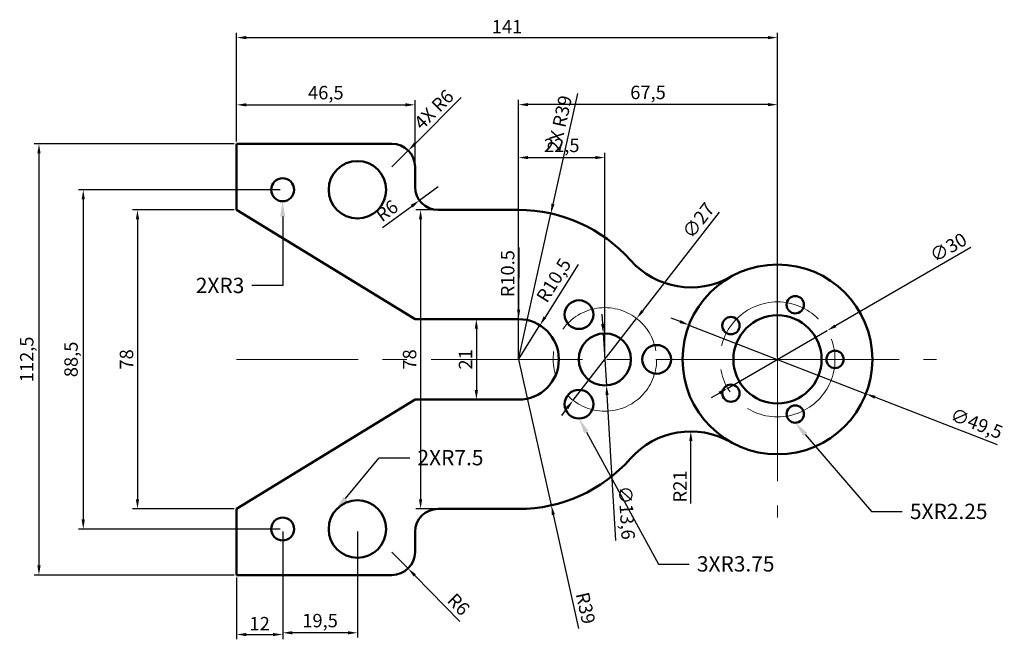
# Model space of a CAD drawing. Units: millimetres. Extents: x 3708 to 3964, y 1647 to 1809.
import ezdxf
from ezdxf import colors
from ezdxf.entities.mleader import LeaderData, LeaderLine
from ezdxf.math import Vec2, Vec3

# ---------------------------------------------------------------- set-up
doc = ezdxf.new("R2010")
doc.units = ezdxf.units.MM
doc.linetypes.add('CENTER', pattern=[50.8, 31.75, -6.35, 6.35, -6.35])
for name, color, linetype, lineweight in [('M-CNTR', 1, 'CENTER', 18), ('M-DIMS', 120, 'Continuous', 25), ('M-OUTL', 7, 'Continuous', 50)]:
    doc.layers.add(name, color=color, linetype=linetype, lineweight=lineweight)
doc.styles.get("Standard").update_dxf_attribs({"font": 'arial.ttf'})
doc.dimstyles.new('ISO-25', dxfattribs={"dimtxt": 3.5, "dimasz": 2.5, "dimexe": 1.25, "dimexo": 0.625, "dimtad": 1, "dimtxsty": 'Standard', "dimcen": 2.5, "dimadec": 0, "dimazin": 0, "dimtfac": 1, "dimtmove": 0, "dimatfit": 3, "dimfxl": 1, "dimarcsym": 0})

# ---------------------------------------------------------------- blocks, each defined once
blk = doc.blocks.new('*D1')
at = {"layer": 'Defpoints', "color": 0, "transparency": 16777216}
for p in [(3764.07, 1776.41), (3712.53, 1663.91), (3764.07, 1663.91)]:
    blk.add_point(p, dxfattribs=at)
at = {"layer": 'M-DIMS', "color": 0, "lineweight": -2, "transparency": 16777216}
for p, q in [((3763.44, 1776.41), (3711.28, 1776.41)), ((3712.53, 1773.91), (3712.53, 1666.41)), ((3763.44, 1663.91), (3711.28, 1663.91))]:
    blk.add_line(p, q, dxfattribs=at)
at = {"layer": 'M-DIMS', "color": 0, "transparency": 16777216}
for points in [[(3712.12, 1773.91), (3712.95, 1773.91), (3712.53, 1776.41)], [(3712.12, 1666.41), (3712.95, 1666.41), (3712.53, 1663.91)]]:
    blk.add_solid(points, dxfattribs=at)
at = {"layer": 'M-DIMS', "color": 0, "transparency": 16777216, "insert": (3709.8, 1720.16), "char_height": 3.5, "attachment_point": 5, "rotation": 90}
blk.add_mtext('112,5', dxfattribs=at)
blk = doc.blocks.new('*D2')
at = {"layer": 'Defpoints', "color": 0, "transparency": 16777216}
for p in [(3776.07, 1764.41), (3724.08, 1675.91), (3776.07, 1675.91)]:
    blk.add_point(p, dxfattribs=at)
at = {"layer": 'M-DIMS', "color": 0, "lineweight": -2, "transparency": 16777216}
for p, q in [((3775.44, 1764.41), (3722.83, 1764.41)), ((3724.08, 1761.91), (3724.08, 1678.41)), ((3775.44, 1675.91), (3722.83, 1675.91))]:
    blk.add_line(p, q, dxfattribs=at)
at = {"layer": 'M-DIMS', "color": 0, "transparency": 16777216}
for points in [[(3723.66, 1761.91), (3724.49, 1761.91), (3724.08, 1764.41)], [(3723.66, 1678.41), (3724.49, 1678.41), (3724.08, 1675.91)]]:
    blk.add_solid(points, dxfattribs=at)
at = {"layer": 'M-DIMS', "color": 0, "transparency": 16777216, "insert": (3721.35, 1720.16), "char_height": 3.5, "attachment_point": 5, "rotation": 90}
blk.add_mtext('88,5', dxfattribs=at)
blk = doc.blocks.new('*D3')
at = {"layer": 'Defpoints', "color": 0, "transparency": 16777216}
for p in [(3764.07, 1759.16), (3738.21, 1681.16), (3764.07, 1681.16)]:
    blk.add_point(p, dxfattribs=at)
at = {"layer": 'M-DIMS', "color": 0, "lineweight": -2, "transparency": 16777216}
for p, q in [((3763.44, 1759.16), (3736.96, 1759.16)), ((3738.21, 1756.66), (3738.21, 1683.66)), ((3763.44, 1681.16), (3736.96, 1681.16))]:
    blk.add_line(p, q, dxfattribs=at)
at = {"layer": 'M-DIMS', "color": 0, "transparency": 16777216}
for points in [[(3737.8, 1756.66), (3738.63, 1756.66), (3738.21, 1759.16)], [(3737.8, 1683.66), (3738.63, 1683.66), (3738.21, 1681.16)]]:
    blk.add_solid(points, dxfattribs=at)
at = {"layer": 'M-DIMS', "color": 0, "transparency": 16777216, "insert": (3735.8, 1720.16), "char_height": 3.5, "attachment_point": 5, "rotation": 90}
blk.add_mtext('78', dxfattribs=at)
blk = doc.blocks.new('*D4')
at = {"layer": 'Defpoints', "color": 0, "transparency": 16777216}
for p in [(3776.07, 1675.91), (3764.07, 1663.91), (3776.07, 1648.4)]:
    blk.add_point(p, dxfattribs=at)
at = {"layer": 'M-DIMS', "color": 0, "lineweight": -2, "transparency": 16777216}
for p, q in [((3776.07, 1675.28), (3776.07, 1647.15)), ((3764.07, 1663.28), (3764.07, 1647.15)), ((3766.57, 1648.4), (3773.57, 1648.4))]:
    blk.add_line(p, q, dxfattribs=at)
at = {"layer": 'M-DIMS', "color": 0, "transparency": 16777216}
for points in [[(3766.57, 1648.81), (3766.57, 1647.98), (3764.07, 1648.4)], [(3773.57, 1648.81), (3773.57, 1647.98), (3776.07, 1648.4)]]:
    blk.add_solid(points, dxfattribs=at)
at = {"layer": 'M-DIMS', "color": 0, "transparency": 16777216, "insert": (3770.07, 1650.78), "char_height": 3.5, "attachment_point": 5}
blk.add_mtext('12', dxfattribs=at)
blk = doc.blocks.new('*D5')
at = {"layer": 'Defpoints', "color": 0, "transparency": 16777216}
for p in [(3776.07, 1675.91), (3795.57, 1675.91), (3776.07, 1648.85)]:
    blk.add_point(p, dxfattribs=at)
at = {"layer": 'M-DIMS', "color": 0, "lineweight": -2, "transparency": 16777216}
for p, q in [((3776.07, 1675.28), (3776.07, 1647.6)), ((3795.57, 1675.28), (3795.57, 1647.6)), ((3793.07, 1648.85), (3778.57, 1648.85))]:
    blk.add_line(p, q, dxfattribs=at)
at = {"layer": 'M-DIMS', "color": 0, "transparency": 16777216}
for points in [[(3778.57, 1649.27), (3778.57, 1648.43), (3776.07, 1648.85)], [(3793.07, 1649.27), (3793.07, 1648.43), (3795.57, 1648.85)]]:
    blk.add_solid(points, dxfattribs=at)
at = {"layer": 'M-DIMS', "color": 0, "transparency": 16777216, "insert": (3785.82, 1651.58), "char_height": 3.5, "attachment_point": 5}
blk.add_mtext('19,5', dxfattribs=at)
blk = doc.blocks.new('*D6')
at = {"layer": 'Defpoints', "color": 0, "transparency": 16777216}
for p in [(3816.57, 1759.16), (3812.03, 1681.16), (3816.57, 1681.16)]:
    blk.add_point(p, dxfattribs=at)
at = {"layer": 'M-DIMS', "color": 0, "lineweight": -2, "transparency": 16777216}
for p, q in [((3815.94, 1759.16), (3810.78, 1759.16)), ((3812.03, 1756.66), (3812.03, 1683.66)), ((3815.94, 1681.16), (3810.78, 1681.16))]:
    blk.add_line(p, q, dxfattribs=at)
at = {"layer": 'M-DIMS', "color": 0, "transparency": 16777216}
for points in [[(3811.61, 1756.66), (3812.44, 1756.66), (3812.03, 1759.16)], [(3811.61, 1683.66), (3812.44, 1683.66), (3812.03, 1681.16)]]:
    blk.add_solid(points, dxfattribs=at)
at = {"layer": 'M-DIMS', "color": 0, "transparency": 16777216, "insert": (3809.61, 1720.16), "char_height": 3.5, "attachment_point": 5, "rotation": 90}
blk.add_mtext('78', dxfattribs=at)
blk = doc.blocks.new('*D7')
at = {"layer": 'Defpoints', "color": 0, "transparency": 16777216}
for p in [(3824.07, 1730.66), (3824.07, 1709.66), (3826.57, 1709.66)]:
    blk.add_point(p, dxfattribs=at)
at = {"layer": 'M-DIMS', "color": 0, "lineweight": -2, "transparency": 16777216}
for p, q in [((3824.69, 1730.66), (3827.82, 1730.66)), ((3826.57, 1728.16), (3826.57, 1712.16)), ((3824.69, 1709.66), (3827.82, 1709.66))]:
    blk.add_line(p, q, dxfattribs=at)
at = {"layer": 'M-DIMS', "color": 0, "transparency": 16777216}
for points in [[(3826.15, 1728.16), (3826.99, 1728.16), (3826.57, 1730.66)], [(3826.15, 1712.16), (3826.99, 1712.16), (3826.57, 1709.66)]]:
    blk.add_solid(points, dxfattribs=at)
at = {"layer": 'M-DIMS', "color": 0, "transparency": 16777216, "insert": (3824.19, 1720.16), "char_height": 3.5, "attachment_point": 5, "rotation": 90}
blk.add_mtext('21', dxfattribs=at)
blk = doc.blocks.new('*D8')
at = {"layer": 'Defpoints', "color": 0, "transparency": 16777216}
for p in [(3810.57, 1786.56), (3764.07, 1776.41), (3810.57, 1767.78)]:
    blk.add_point(p, dxfattribs=at)
at = {"layer": 'M-DIMS', "color": 0, "lineweight": -2, "transparency": 16777216}
for p, q in [((3764.07, 1777.03), (3764.07, 1787.81)), ((3810.57, 1768.41), (3810.57, 1787.81)), ((3766.57, 1786.56), (3808.07, 1786.56))]:
    blk.add_line(p, q, dxfattribs=at)
at = {"layer": 'M-DIMS', "color": 0, "transparency": 16777216}
for points in [[(3766.57, 1786.98), (3766.57, 1786.15), (3764.07, 1786.56)], [(3808.07, 1786.98), (3808.07, 1786.15), (3810.57, 1786.56)]]:
    blk.add_solid(points, dxfattribs=at)
at = {"layer": 'M-DIMS', "color": 0, "transparency": 16777216, "insert": (3787.32, 1789.29), "char_height": 3.5, "attachment_point": 5}
blk.add_mtext('46,5', dxfattribs=at)
blk = doc.blocks.new('*D9')
at = {"layer": 'Defpoints', "color": 0, "transparency": 16777216}
for p in [(3905.07, 1804.1), (3764.07, 1776.41), (3905.07, 1720.16)]:
    blk.add_point(p, dxfattribs=at)
at = {"layer": 'M-DIMS', "color": 0, "lineweight": -2, "transparency": 16777216}
for p, q in [((3764.07, 1777.03), (3764.07, 1805.35)), ((3905.07, 1720.78), (3905.07, 1805.35)), ((3766.57, 1804.1), (3902.57, 1804.1))]:
    blk.add_line(p, q, dxfattribs=at)
at = {"layer": 'M-DIMS', "color": 0, "transparency": 16777216}
for points in [[(3766.57, 1804.51), (3766.57, 1803.68), (3764.07, 1804.1)], [(3902.57, 1804.51), (3902.57, 1803.68), (3905.07, 1804.1)]]:
    blk.add_solid(points, dxfattribs=at)
at = {"layer": 'M-DIMS', "color": 0, "transparency": 16777216, "insert": (3834.57, 1806.48), "char_height": 3.5, "attachment_point": 5}
blk.add_mtext('141', dxfattribs=at)
blk = doc.blocks.new('*D10')
at = {"layer": 'Defpoints', "color": 0, "transparency": 16777216}
for p in [(3837.57, 1786.62), (3837.57, 1720.16), (3905.07, 1720.16)]:
    blk.add_point(p, dxfattribs=at)
at = {"layer": 'M-DIMS', "color": 0, "lineweight": -2, "transparency": 16777216}
for p, q in [((3837.57, 1720.78), (3837.57, 1787.87)), ((3905.07, 1720.78), (3905.07, 1787.87)), ((3902.57, 1786.62), (3840.07, 1786.62))]:
    blk.add_line(p, q, dxfattribs=at)
at = {"layer": 'M-DIMS', "color": 0, "transparency": 16777216}
for points in [[(3840.07, 1787.04), (3840.07, 1786.2), (3837.57, 1786.62)], [(3902.57, 1787.04), (3902.57, 1786.2), (3905.07, 1786.62)]]:
    blk.add_solid(points, dxfattribs=at)
at = {"layer": 'M-DIMS', "color": 0, "transparency": 16777216, "insert": (3871.32, 1789.35), "char_height": 3.5, "attachment_point": 5}
blk.add_mtext('67,5', dxfattribs=at)
blk = doc.blocks.new('*D11')
at = {"layer": 'Defpoints', "color": 0, "transparency": 16777216}
for p in [(3860.07, 1772.81), (3837.57, 1720.16), (3860.07, 1720.16)]:
    blk.add_point(p, dxfattribs=at)
at = {"layer": 'M-DIMS', "color": 0, "lineweight": -2, "transparency": 16777216}
for p, q in [((3837.57, 1720.78), (3837.57, 1774.06)), ((3860.07, 1720.78), (3860.07, 1774.06)), ((3840.07, 1772.81), (3857.57, 1772.81))]:
    blk.add_line(p, q, dxfattribs=at)
at = {"layer": 'M-DIMS', "color": 0, "transparency": 16777216}
for points in [[(3840.07, 1773.22), (3840.07, 1772.39), (3837.57, 1772.81)], [(3857.57, 1773.22), (3857.57, 1772.39), (3860.07, 1772.81)]]:
    blk.add_solid(points, dxfattribs=at)
at = {"layer": 'M-DIMS', "color": 0, "transparency": 16777216, "insert": (3848.82, 1775.53), "char_height": 3.5, "attachment_point": 5}
blk.add_mtext('22,5', dxfattribs=at)
blk = doc.blocks.new('*D12')
at = {"layer": 'Defpoints', "color": 0, "transparency": 16777216}
for p in [(3816.57, 1765.16), (3811.73, 1761.62)]:
    blk.add_point(p, dxfattribs=at)
at = {"layer": 'M-DIMS', "color": 0, "lineweight": -2, "transparency": 16777216}
for p, q in [((3816.57, 1765.16), (3811.73, 1761.62)), ((3802.13, 1754.6), (3809.71, 1760.14))]:
    blk.add_line(p, q, dxfattribs=at)
at = {"layer": 'M-DIMS', "color": 0, "transparency": 16777216}
blk.add_solid([(3809.46, 1760.48), (3809.96, 1759.8), (3811.73, 1761.62)], dxfattribs=at)
at = {"layer": 'M-DIMS', "color": 0, "transparency": 16777216, "insert": (3803.49, 1758.58), "char_height": 3.5, "attachment_point": 5, "rotation": 36.1895}
blk.add_mtext('R6', dxfattribs=at)
blk = doc.blocks.new('*D13')
at = {"layer": 'Defpoints', "color": 0, "transparency": 16777216}
for p in [(3804.57, 1669.91), (3808.77, 1665.62)]:
    blk.add_point(p, dxfattribs=at)
at = {"layer": 'M-DIMS', "color": 0, "lineweight": -2, "transparency": 16777216}
for p, q in [((3804.57, 1669.91), (3808.77, 1665.62)), ((3822.28, 1651.8), (3810.51, 1663.83))]:
    blk.add_line(p, q, dxfattribs=at)
at = {"layer": 'M-DIMS', "color": 0, "transparency": 16777216}
blk.add_solid([(3810.81, 1664.12), (3810.22, 1663.54), (3808.77, 1665.62)], dxfattribs=at)
at = {"layer": 'M-DIMS', "color": 0, "transparency": 16777216, "insert": (3821.6, 1655.95), "char_height": 3.5, "attachment_point": 5, "rotation": 314.3673}
blk.add_mtext('R6', dxfattribs=at)
blk = doc.blocks.new('*D14')
at = {"layer": 'Defpoints', "color": 0, "transparency": 16777216}
for p in [(3837.57, 1720.16), (3846.11, 1682.11)]:
    blk.add_point(p, dxfattribs=at)
at = {"layer": 'M-DIMS', "color": 0, "lineweight": -2, "transparency": 16777216}
for p, q in [((3837.57, 1720.16), (3846.11, 1682.11)), ((3853.32, 1649.97), (3846.66, 1679.67))]:
    blk.add_line(p, q, dxfattribs=at)
at = {"layer": 'M-DIMS', "color": 0, "transparency": 16777216}
blk.add_solid([(3847.06, 1679.76), (3846.25, 1679.58), (3846.11, 1682.11)], dxfattribs=at)
at = {"layer": 'M-DIMS', "color": 0, "transparency": 16777216, "insert": (3854.62, 1655.19), "char_height": 3.5, "attachment_point": 5, "rotation": 282.6469}
blk.add_mtext('R39', dxfattribs=at)
blk = doc.blocks.new('*D15')
at = {"layer": 'Defpoints', "color": 0, "transparency": 16777216}
for p in [(3882.48, 1701.37), (3882.48, 1680.37)]:
    blk.add_point(p, dxfattribs=at)
at = {"layer": 'M-DIMS', "color": 0, "lineweight": -2, "transparency": 16777216}
blk.add_line((3882.48, 1682.54), (3882.48, 1698.87), dxfattribs=at)
at = {"layer": 'M-DIMS', "color": 0, "transparency": 16777216}
blk.add_solid([(3882.07, 1698.87), (3882.9, 1698.87), (3882.48, 1701.37)], dxfattribs=at)
at = {"layer": 'M-DIMS', "color": 0, "transparency": 16777216, "insert": (3880.1, 1687.01), "char_height": 3.5, "attachment_point": 5, "rotation": 90}
blk.add_mtext('R21', dxfattribs=at)
blk = doc.blocks.new('*D16')
at = {"layer": 'Defpoints', "color": 0, "transparency": 16777216}
for p in [(3843.14, 1729.06), (3837.57, 1720.16)]:
    blk.add_point(p, dxfattribs=at)
at = {"layer": 'M-DIMS', "color": 0, "lineweight": -2, "transparency": 16777216}
for p, q in [((3853.07, 1744.93), (3844.47, 1731.18)), ((3837.57, 1720.16), (3843.14, 1729.06))]:
    blk.add_line(p, q, dxfattribs=at)
at = {"layer": 'M-DIMS', "color": 0, "transparency": 16777216}
blk.add_solid([(3844.11, 1731.4), (3844.82, 1730.96), (3843.14, 1729.06)], dxfattribs=at)
at = {"layer": 'M-DIMS', "color": 0, "transparency": 16777216, "insert": (3847.12, 1740.56), "char_height": 3.5, "attachment_point": 5, "rotation": 57.9597}
blk.add_mtext('R10,5', dxfattribs=at)
blk = doc.blocks.new('*D17')
at = {"layer": 'Defpoints', "color": 0, "transparency": 16777216}
for p in [(3882, 1729.12), (3928.14, 1711.2)]:
    blk.add_point(p, dxfattribs=at)
at = {"layer": 'M-DIMS', "color": 0, "lineweight": -2, "transparency": 16777216}
for p, q in [((3879.67, 1730.02), (3877.34, 1730.93)), ((3882, 1729.12), (3928.14, 1711.2)), ((3962.43, 1697.88), (3930.47, 1710.29))]:
    blk.add_line(p, q, dxfattribs=at)
at = {"layer": 'M-DIMS', "color": 0, "transparency": 16777216}
for points in [[(3879.82, 1730.41), (3879.52, 1729.64), (3882, 1729.12)], [(3930.62, 1710.68), (3930.32, 1709.91), (3928.14, 1711.2)]]:
    blk.add_solid(points, dxfattribs=at)
at = {"layer": 'M-DIMS', "color": 0, "transparency": 16777216, "insert": (3956.83, 1703.05), "char_height": 3.5, "attachment_point": 5, "rotation": 338.775}
blk.add_mtext('∅49,5', dxfattribs=at)
blk = doc.blocks.new('*D18')
at = {"layer": 'Defpoints', "color": 0, "transparency": 16777216}
for p in [(3918.05, 1727.68), (3892.09, 1712.64)]:
    blk.add_point(p, dxfattribs=at)
at = {"layer": 'M-DIMS', "color": 0, "lineweight": -2, "transparency": 16777216}
for p, q in [((3955.45, 1749.34), (3920.21, 1728.93)), ((3892.09, 1712.64), (3918.05, 1727.68)), ((3889.93, 1711.39), (3887.76, 1710.14))]:
    blk.add_line(p, q, dxfattribs=at)
at = {"layer": 'M-DIMS', "color": 0, "transparency": 16777216}
for points in [[(3920, 1729.29), (3920.42, 1728.57), (3918.05, 1727.68)], [(3889.72, 1711.75), (3890.14, 1711.03), (3892.09, 1712.64)]]:
    blk.add_solid(points, dxfattribs=at)
at = {"layer": 'M-DIMS', "color": 0, "transparency": 16777216, "insert": (3949.84, 1748.99), "char_height": 3.5, "attachment_point": 5, "rotation": 30.0783}
blk.add_mtext('∅30', dxfattribs=at)
blk = doc.blocks.new('*D19')
at = {"layer": 'Defpoints', "color": 0, "transparency": 16777216}
for p in [(3868.34, 1730.83), (3851.8, 1709.49)]:
    blk.add_point(p, dxfattribs=at)
at = {"layer": 'M-DIMS', "color": 0, "lineweight": -2, "transparency": 16777216}
for p, q in [((3889.87, 1758.57), (3869.88, 1732.8)), ((3851.8, 1709.49), (3868.34, 1730.83)), ((3850.26, 1707.52), (3848.73, 1705.54))]:
    blk.add_line(p, q, dxfattribs=at)
at = {"layer": 'M-DIMS', "color": 0, "transparency": 16777216}
for points in [[(3869.55, 1733.06), (3870.21, 1732.55), (3868.34, 1730.83)], [(3849.93, 1707.77), (3850.59, 1707.26), (3851.8, 1709.49)]]:
    blk.add_solid(points, dxfattribs=at)
at = {"layer": 'M-DIMS', "color": 0, "transparency": 16777216, "insert": (3884.8, 1756.13), "char_height": 3.5, "attachment_point": 5, "rotation": 52.1995}
blk.add_mtext('∅27', dxfattribs=at)
blk = doc.blocks.new('*D20')
at = {"layer": 'Defpoints', "color": 0, "transparency": 16777216}
for p in [(3859.65, 1726.95), (3860.49, 1713.37)]:
    blk.add_point(p, dxfattribs=at)
at = {"layer": 'M-DIMS', "color": 0, "lineweight": -2, "transparency": 16777216}
for p, q in [((3859.5, 1729.44), (3859.35, 1731.94)), ((3859.65, 1726.95), (3860.49, 1713.37)), ((3862.96, 1672.92), (3860.64, 1710.88))]:
    blk.add_line(p, q, dxfattribs=at)
at = {"layer": 'M-DIMS', "color": 0, "transparency": 16777216}
for points in [[(3859.92, 1729.47), (3859.09, 1729.42), (3859.65, 1726.95)], [(3861.05, 1710.9), (3860.22, 1710.85), (3860.49, 1713.37)]]:
    blk.add_solid(points, dxfattribs=at)
at = {"layer": 'M-DIMS', "color": 0, "transparency": 16777216, "insert": (3865.31, 1680.15), "char_height": 3.5, "attachment_point": 5, "rotation": 273.5032}
blk.add_mtext('∅13,6', dxfattribs=at)
blk = doc.blocks.new('FORK-HOLE-PAIR-D6-D15')
for centre, radius in [((19.5, 0), 7.5), ((0, 0), 3)]:
    blk.add_circle(centre, radius)
blk = doc.blocks.new('HOLE-D7_5')
blk.add_circle((0, 0), 3.75)
blk = doc.blocks.new('HOLE-D4_5')
blk.add_circle((0, 0), 2.25)
blk = doc.blocks.new('*D24')
at = {"layer": 'Defpoints', "color": 0, "transparency": 16777216}
for p in [(3846, 1758.24), (3837.57, 1720.16)]:
    blk.add_point(p, dxfattribs=at)
at = {"layer": 'M-DIMS', "color": 0, "lineweight": -2, "transparency": 16777216}
for p, q in [((3852.92, 1789.48), (3846.54, 1760.68)), ((3837.57, 1720.16), (3846, 1758.24))]:
    blk.add_line(p, q, dxfattribs=at)
at = {"layer": 'M-DIMS', "color": 0, "transparency": 16777216}
blk.add_solid([(3846.13, 1760.77), (3846.95, 1760.59), (3846, 1758.24)], dxfattribs=at)
at = {"layer": 'M-DIMS', "color": 0, "transparency": 16777216, "insert": (3848.7, 1781.61), "char_height": 3.5, "attachment_point": 5, "rotation": 77.5173}
blk.add_mtext('2X R39', dxfattribs=at)
blk = doc.blocks.new('*D25')
at = {"layer": 'Defpoints', "color": 0, "transparency": 16777216}
for p in [(3808.81, 1774.65), (3804.57, 1770.41)]:
    blk.add_point(p, dxfattribs=at)
at = {"layer": 'M-DIMS', "color": 0, "lineweight": -2, "transparency": 16777216}
for p, q in [((3822.64, 1788.48), (3810.58, 1776.42)), ((3804.57, 1770.41), (3808.81, 1774.65))]:
    blk.add_line(p, q, dxfattribs=at)
at = {"layer": 'M-DIMS', "color": 0, "transparency": 16777216}
blk.add_solid([(3810.29, 1776.71), (3810.87, 1776.13), (3808.81, 1774.65)], dxfattribs=at)
at = {"layer": 'M-DIMS', "color": 0, "transparency": 16777216, "insert": (3815.79, 1785.04), "char_height": 3.5, "attachment_point": 5, "rotation": 45.0017}
blk.add_mtext('4X R6', dxfattribs=at)
blk = doc.blocks.new('*D26')
at = {"layer": 'Defpoints', "color": 0, "transparency": 16777216}
for p in [(3837.58, 1730.66), (3837.57, 1720.16)]:
    blk.add_point(p, dxfattribs=at)
at = {"layer": 'M-DIMS', "color": 0, "lineweight": -2, "transparency": 16777216}
for p, q in [((3837.6, 1749.38), (3837.58, 1733.16)), ((3837.57, 1720.16), (3837.58, 1730.66))]:
    blk.add_line(p, q, dxfattribs=at)
at = {"layer": 'M-DIMS', "color": 0, "transparency": 16777216}
blk.add_solid([(3837.17, 1733.16), (3838, 1733.16), (3837.58, 1730.66)], dxfattribs=at)
at = {"layer": 'M-DIMS', "color": 0, "transparency": 16777216, "insert": (3835.18, 1742.52), "char_height": 3.5, "attachment_point": 5, "rotation": 89.9446}
blk.add_mtext('R10.5', dxfattribs=at)

msp = doc.modelspace()

# ---------------------------------------------------------------- linework, layer by layer
at = {"layer": 'M-CNTR'}
for p, q in [((3905.07, 1720.16), (3905.07, 1764.926)), ((3846.57, 1720.16), (3764.07, 1720.16)), ((3905.07, 1720.16), (3837.57, 1720.16)), ((3905.07, 1720.16), (3946.49, 1720.16)), ((3905.07, 1720.16), (3905.07, 1678.941))]:
    msp.add_line(p, q, dxfattribs=at)
for centre, radius in [((3860.07, 1720.16), 13.5), ((3905.07, 1720.16), 15)]:
    msp.add_circle(centre, radius, dxfattribs=at)
at = {"layer": 'M-OUTL'}
for p, q in [((3764.07, 1759.16), (3764.07, 1776.41)), ((3764.07, 1776.41), (3804.57, 1776.41)), ((3810.57, 1770.41), (3810.57, 1765.16)), ((3764.07, 1759.16), (3810.57, 1730.66)), ((3837.57, 1759.16), (3816.57, 1759.16)), ((3837.57, 1730.66), (3810.57, 1730.66)), ((3810.57, 1709.66), (3764.07, 1681.16)), ((3810.57, 1709.66), (3837.57, 1709.66)), ((3764.07, 1681.16), (3764.07, 1663.91)), ((3837.57, 1681.16), (3816.57, 1681.16)), ((3810.57, 1669.91), (3810.57, 1675.16)), ((3764.07, 1663.91), (3804.57, 1663.91))]:
    msp.add_line(p, q, dxfattribs=at)
for centre, radius in [((3905.07, 1720.16), 24.75), ((3905.07, 1720.16), 11.5), ((3860.07, 1720.16), 6.8)]:
    msp.add_circle(centre, radius, dxfattribs=at)
for centre, radius, start, end in [((3804.57, 1770.41), 6, 0, 90), ((3816.57, 1765.16), 6, 180, 270), ((3837.57, 1720.16), 39, 41.53579, 90), ((3882.482, 1759.945), 21, 221.53579, 299.58511), ((3837.57, 1720.16), 10.5, 270, 90), ((3882.482, 1680.374), 21, 60.41489, 138.46421), ((3837.57, 1720.16), 39, 270, 318.46421), ((3816.57, 1675.16), 6, 90, 180), ((3804.57, 1669.91), 6, 270, 0)]:
    msp.add_arc(centre, radius, start, end, dxfattribs=at)

# ---------------------------------------------------------------- block references
for name, p in [('FORK-HOLE-PAIR-D6-D15', (3776.07, 1764.41)), ('HOLE-D7_5', (3853.32, 1731.851)), ('HOLE-D4_5', (3909.705, 1734.425)), ('HOLE-D4_5', (3892.935, 1728.976)), ('HOLE-D7_5', (3873.57, 1720.16)), ('HOLE-D4_5', (3920.07, 1720.16)), ('HOLE-D4_5', (3892.935, 1711.343)), ('HOLE-D7_5', (3853.32, 1708.468)), ('HOLE-D4_5', (3909.705, 1705.894)), ('FORK-HOLE-PAIR-D6-D15', (3776.07, 1675.91))]:
    msp.add_blockref(name, p, dxfattribs=at)

# ---------------------------------------------------------------- dimensions: what is measured, and where the dimension line sits
at = {"layer": 'M-DIMS'}
for base, p1, p2, picture, middle in [((3905.07, 1804.098), (3764.07, 1776.41), (3905.07, 1720.16), '*D9', (3834.57, 1806.48)), ((3810.57, 1786.564), (3764.07, 1776.41), (3810.57, 1767.785), '*D8', (3787.32, 1789.292)), ((3837.57, 1786.62), (3905.07, 1720.16), (3837.57, 1720.16), '*D10', (3871.32, 1789.348)), ((3860.07, 1772.806), (3837.57, 1720.16), (3860.07, 1720.16), '*D11', (3848.82, 1775.534)), ((3776.07, 1648.397), (3764.07, 1663.91), (3776.07, 1675.91), '*D4', (3770.07, 1650.779)), ((3776.07, 1648.849), (3795.57, 1675.91), (3776.07, 1675.91), '*D5', (3785.82, 1651.577))]:
    dim = msp.add_linear_dim(base=base, p1=p1, p2=p2, dimstyle='ISO-25', override={"dimclrd": 0, "dimclre": 0, "dimclrt": 0}, dxfattribs=at)
    dim.commit()
    dim.dimension.update_dxf_attribs({"geometry": picture, "text_midpoint": middle})
dim = msp.add_radius_dim(center=(3804.57, 1770.41), mpoint=(3808.812, 1774.652), text='4X <>', dimstyle='ISO-25', override={"dimdec": 0, "dimlfac": 1, "dimrnd": 0, "dimzin": 0, "dimdsep": 46, "dimlunit": 2}, dxfattribs=at)
dim.commit()
dim.dimension.update_dxf_attribs({"geometry": '*D25', "text_midpoint": (3815.787, 1785.039)})
dim = msp.add_radius_dim(center=(3837.57, 1720.16), mpoint=(3845.999, 1758.238), text='2X <>', dimstyle='ISO-25', override={"dimdec": 0, "dimlfac": 1, "dimrnd": 0, "dimzin": 0, "dimdsep": 46, "dimlunit": 2}, dxfattribs=at)
dim.commit()
dim.dimension.update_dxf_attribs({"geometry": '*D24', "text_midpoint": (3851.057, 1781.085), "dimtype": 164})
for base, p1, p2, picture, middle in [((3712.532, 1663.91), (3764.07, 1776.41), (3764.07, 1663.91), '*D1', (3709.804, 1720.16)), ((3724.076, 1675.91), (3776.07, 1764.41), (3776.07, 1675.91), '*D2', (3721.348, 1720.16)), ((3738.212, 1681.16), (3764.07, 1759.16), (3764.07, 1681.16), '*D3', (3735.8, 1720.16)), ((3812.027, 1681.16), (3816.57, 1759.16), (3816.57, 1681.16), '*D6', (3809.615, 1720.16)), ((3826.57, 1709.66), (3824.07, 1730.66), (3824.07, 1709.66), '*D7', (3824.188, 1720.16))]:
    dim = msp.add_linear_dim(base=base, p1=p1, p2=p2, angle=90, dimstyle='ISO-25', override={"dimclrd": 0, "dimclre": 0, "dimclrt": 0}, dxfattribs=at)
    dim.commit()
    dim.dimension.update_dxf_attribs({"geometry": picture, "text_midpoint": middle})
for center, mpoint, override, picture, middle in [((3816.57, 1765.16), (3811.727, 1761.617), {"dimclrd": 0, "dimclre": 0, "dimclrt": 0}, '*D12', (3803.487, 1758.577)), ((3837.57, 1720.16), (3837.58, 1730.66), {"dimdec": 1, "dimlfac": 1, "dimrnd": 0, "dimzin": 0, "dimdsep": 46, "dimlunit": 2}, '*D26', (3835.179, 1742.521)), ((3837.57, 1720.16), (3843.14, 1729.06), {"dimclrd": 0, "dimclre": 0, "dimclrt": 0}, '*D16', (3847.119, 1740.56))]:
    dim = msp.add_radius_dim(center=center, mpoint=mpoint, dimstyle='ISO-25', override=override, dxfattribs=at)
    dim.commit()
    dim.dimension.update_dxf_attribs({"geometry": picture, "text_midpoint": middle})
for p1, p2, picture, middle in [((3851.796, 1709.493), (3868.344, 1730.827), '*D19', (3886.781, 1754.594)), ((3892.09, 1712.642), (3918.05, 1727.677), '*D18', (3951.102, 1746.82)), ((3859.654, 1726.947), (3860.485, 1713.372), '*D20', (3862.53, 1679.975)), ((3881.999, 1729.12), (3928.141, 1711.199), '*D17', (3955.822, 1700.449))]:
    dim = msp.add_diameter_dim_2p(p1=p1, p2=p2, dimstyle='ISO-25', override={"dimclrd": 0, "dimclre": 0, "dimclrt": 0}, dxfattribs=at)
    dim.commit()
    dim.dimension.update_dxf_attribs({"geometry": picture, "text_midpoint": middle, "dimtype": 163})
for center, mpoint, picture, middle in [((3837.57, 1720.16), (3846.109, 1682.106), '*D14', (3852.265, 1654.667)), ((3882.482, 1680.374), (3882.482, 1701.374), '*D15', (3882.482, 1687.009)), ((3804.57, 1669.91), (3808.765, 1665.62), '*D13', (3819.873, 1654.264))]:
    dim = msp.add_radius_dim(center=center, mpoint=mpoint, dimstyle='ISO-25', override={"dimclrd": 0, "dimclre": 0, "dimclrt": 0}, dxfattribs=at)
    dim.commit()
    dim.dimension.update_dxf_attribs({"geometry": picture, "text_midpoint": middle, "dimtype": 164})

# ---------------------------------------------------------------- leaders
ml = msp.add_multileader_mtext('Standard', dxfattribs=at)
ml.set_content('2XR3', color=256)
ml.set_leader_properties()
ml.build(insert=Vec2(0, 0))
ctx = ml.context
ctx.base_point, ctx.plane_origin = Vec3(3750.509, 1739.42), Vec3(3776.07, 1761.41)
ctx.text_align_type = 2
notes = []
notes.append((ctx, [(0, (1, 1, 0), (3776.07, 1739.42), (-1, 0), 8, [(0, [(3776.07, 1761.41)], 0, [])])]))
ctx.mtext.insert, ctx.mtext.alignment, ctx.mtext.flow_direction = Vec3(3766.07, 1741.456), 3, 5
ml = msp.add_multileader_mtext('Standard', dxfattribs=at)
ml.set_content('3XR3.75', color=256)
ml.set_leader_properties()
ml.build(insert=Vec2(0, 0))
ctx = ml.context
ctx.base_point, ctx.plane_origin = Vec3(3882.064, 1666.791), Vec3(3853.32, 1704.718)
notes.append((ctx, [(0, (1, 1, 0), (3874.064, 1666.791), (1, 0), 8, [(0, [(3853.32, 1704.718)], 0, [])])]))
ctx.mtext.insert, ctx.mtext.flow_direction = Vec3(3884.064, 1668.827), 5
ml = msp.add_multileader_mtext('Standard', dxfattribs=at)
ml.set_content('5XR2.25', color=256)
ml.set_leader_properties()
ml.build(insert=Vec2(0, 0))
ctx = ml.context
ctx.base_point, ctx.plane_origin = Vec3(3937.608, 1680.482), Vec3(3909.705, 1703.644)
notes.append((ctx, [(0, (1, 1, 0), (3929.608, 1680.482), (1, 0), 8, [(0, [(3909.705, 1703.644)], 0, [])])]))
ctx.mtext.insert, ctx.mtext.flow_direction = Vec3(3939.608, 1682.517), 5
ml = msp.add_multileader_mtext('Standard', dxfattribs=at)
ml.set_content('2XR7.5', color=256)
ml.set_leader_properties()
ml.build(insert=Vec2(0, 0))
ctx = ml.context
ctx.base_point, ctx.plane_origin = Vec3(3809.218, 1694.501), Vec3(3789.86, 1680.773)
notes.append((ctx, [(0, (1, 1, 0), (3801.218, 1694.501), (1, 0), 8, [(0, [(3789.86, 1680.773)], 0, [])])]))
ctx.mtext.insert, ctx.mtext.flow_direction = Vec3(3811.218, 1696.535), 5
for ctx, leaders in notes:
    for number, flags, end, landing, length, lines in leaders:
        leader = LeaderData()
        leader.index, (leader.has_last_leader_line, leader.has_dogleg_vector, leader.attachment_direction) = number, flags
        leader.last_leader_point, leader.dogleg_vector, leader.dogleg_length = Vec3(end), Vec3(landing), length
        for number, points, colour, breaks in lines:
            line = LeaderLine()
            line.index, line.vertices, line.color, line.breaks = number, Vec3.list(points), colors.encode_raw_color(colour), breaks
            leader.lines.append(line)
        ctx.leaders.append(leader)

doc.saveas('drawing.dxf')
